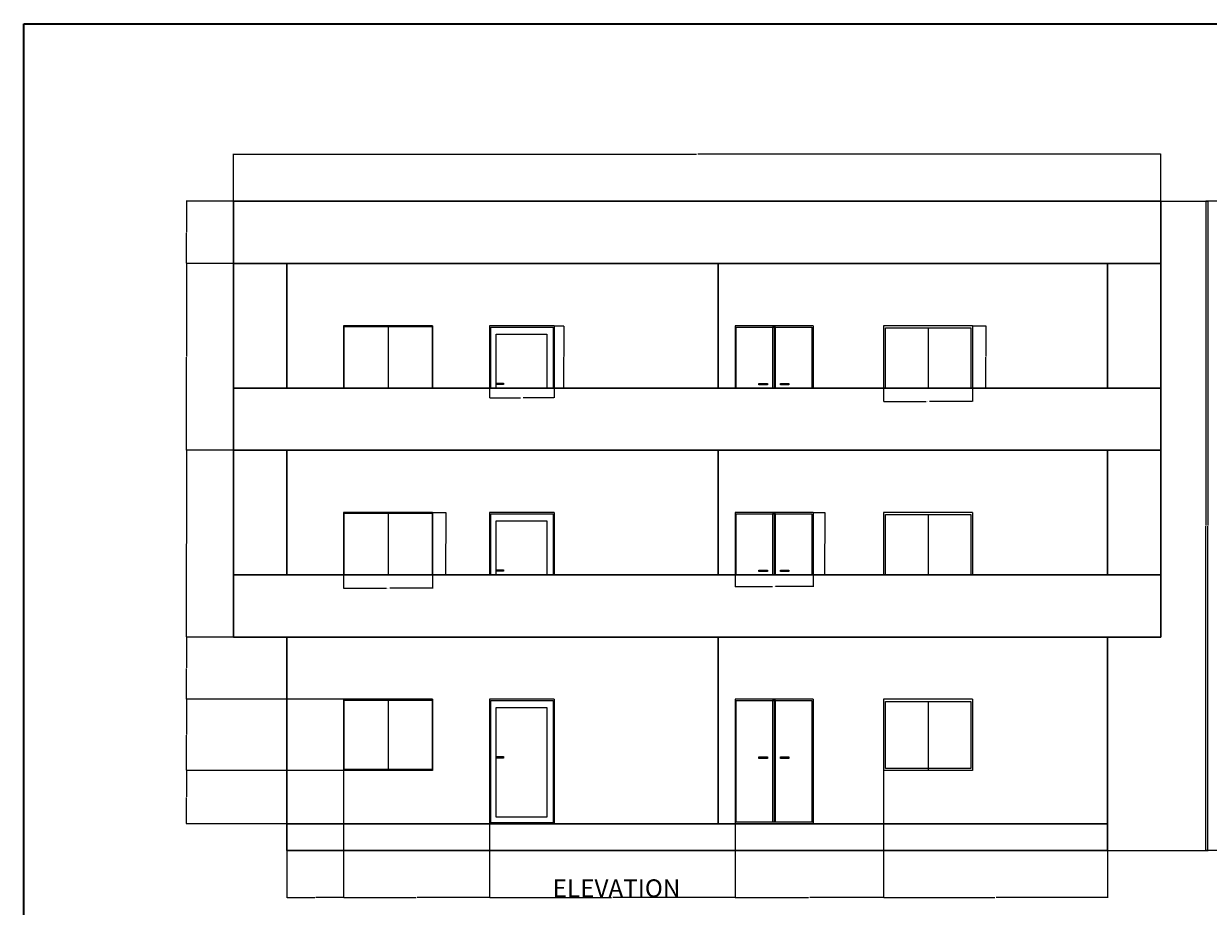
# Model space of a CAD drawing. Units: inches. Extents: x 2014 to 3678, y 870 to 2323.
# Tile 3 of 7: x 2014 to 2813, y 1728 to 2323. Entities that reach past the tile are written whole.
import ezdxf

# ---------------------------------------------------------------- set-up
doc = ezdxf.new("R2010")
doc.units = ezdxf.units.IN
for name, color, linetype, lineweight in [('A-ANNO-DIMS', 2, 'Continuous', 18), ('A-ANNO-TEXT', 7, 'Continuous', 18), ('A-ANNO-TTLB', 7, 'Continuous', 35), ('A-ELEV', 7, 'Continuous', 30), ('A-ELEV-DOOR', 3, 'Continuous', 18), ('A-ELEV-GLAZ', 4, 'Continuous', 18)]:
    doc.layers.add(name, color=color, linetype=linetype, lineweight=lineweight)
doc.styles.get("Standard").update_dxf_attribs({"font": 'arial.ttf'})
doc.dimstyles.get("Standard").update_dxf_attribs({"dimtxt": 0.18, "dimasz": 0.18, "dimexe": 0.18, "dimexo": 0.0625, "dimgap": 0.09, "dimtad": 0, "dimtih": 1, "dimtoh": 1, "dimdec": 4, "dimzin": 0, "dimdsep": 46, "dimtxsty": 'Standard', "dimcen": 0.09, "dimadec": 0, "dimazin": 0, "dimtfac": 1, "dimtdec": 4, "dimtofl": 0, "dimtmove": 0, "dimatfit": 3, "dimfxl": 1, "dimtolj": 1, "dimtzin": 0, "dimarcsym": 0})

# ---------------------------------------------------------------- blocks, each defined once
blk = doc.blocks.new('ELEV-BALCONY-DOOR')
for p, q in [((0, 42), (0, 0)), ((43.48, 42), (0, 42)), ((0, 42), (0, 0)), ((43.48, 42), (0, 42)), ((43.48, 42), (43.48, 0)), ((43.48, 42), (43.48, 0))]:
    blk.add_line(p, q)
for points in [[(0.77, 0), (0.77, 41.09), (42.81, 41.09), (42.81, 0)], [(4.43, 0), (4.43, 36.38), (38.55, 36.38), (38.55, 0)]]:
    blk.add_lwpolyline(points)
blk.add_lwpolyline([(4.43, 3.32), (9.34, 3.32), (9.34, 2.33), (4.43, 2.33)], close=True)
blk = doc.blocks.new('ELEV-BALCONY-DOUBLE-DOOR')
for p, q in [((0, 42), (0, 0)), ((52.71, 42), (0, 42)), ((0, 42), (0, 0)), ((52.71, 42), (0, 42)), ((26.3, 41.16), (25.3, 41.16)), ((25.3, 41.16), (25.3, 0)), ((26.3, 41.16), (26.3, 0)), ((27.3, 41.16), (26.3, 41.16)), ((27.3, 0), (27.3, 41.16)), ((52.71, 42), (52.71, 0)), ((52.71, 42), (52.71, 0))]:
    blk.add_line(p, q)
blk.add_lwpolyline([(0.85, 0), (0.85, 41.16), (51.75, 41.16), (51.75, 0)])
for points in [[(16.11, 3.13), (21.78, 3.13), (21.78, 2.12), (16.11, 2.12)], [(30.59, 3.13), (36.26, 3.13), (36.26, 2.12), (30.59, 2.12)]]:
    blk.add_lwpolyline(points, close=True)
blk = doc.blocks.new('ELEV-BALCONY-WIN-WEST')
for p, q in [((0, 42), (0, 0)), ((60, 42), (0, 42)), ((0, 42), (0, 0)), ((60, 42), (0, 42)), ((30, 42), (30, 0)), ((60, 42), (60, 0)), ((60, 42), (60, 0))]:
    blk.add_line(p, q)
blk.add_lwpolyline([(0.47, 0), (0.47, 41.49), (59.63, 41.49), (59.63, 0)])
blk = doc.blocks.new('ELEV-BALCONY-WIN-EAST')
for p, q in [((0, 42), (0, 0)), ((60, 42), (0, 42)), ((0, 42), (0, 0)), ((60, 42), (0, 42)), ((30.07, 40.6), (30.07, 0)), ((60, 42), (60, 0)), ((60, 42), (60, 0))]:
    blk.add_line(p, q)
blk.add_lwpolyline([(1.35, 0), (1.35, 40.6), (58.8, 40.6), (58.8, 0)])
blk = doc.blocks.new('*D72')
at = {"layer": 'A-ANNO-DIMS', "color": 0, "lineweight": -2, "transparency": 16777216}
for p, q in [((2328.3, 2077.46), (2328.3, 2070.82)), ((2328.48, 2071), (2349.1, 2071)), ((2371.59, 2071), (2350.97, 2071)), ((2371.77, 2077.46), (2371.77, 2070.82))]:
    blk.add_line(p, q, dxfattribs=at)
at = {"layer": 'A-ANNO-DIMS', "color": 0, "transparency": 16777216}
for points in [[(2328.48, 2071.03), (2328.48, 2070.97), (2328.3, 2071)], [(2371.59, 2071.03), (2371.59, 2070.97), (2371.77, 2071)]]:
    blk.add_solid(points, dxfattribs=at)
at = {"layer": 'Defpoints', "color": 0, "transparency": 16777216}
for p in [(2328.3, 2077.52), (2371.77, 2077.52), (2371.77, 2071)]:
    blk.add_point(p, dxfattribs=at)
at = {"layer": 'A-ANNO-DIMS', "color": 0, "transparency": 16777216, "insert": (2350.03, 2071), "char_height": 0.18, "attachment_point": 5}
blk.add_mtext('\\A1;DOOR 43 TYP.', dxfattribs=at)
blk = doc.blocks.new('*D73')
at = {"layer": 'A-ANNO-DIMS', "color": 0, "lineweight": -2, "transparency": 16777216}
for p, q in [((2371.84, 2119.52), (2378.47, 2119.52)), ((2378.29, 2119.34), (2378.29, 2098.7)), ((2378.29, 2077.7), (2378.29, 2098.34)), ((2371.84, 2077.52), (2378.47, 2077.52))]:
    blk.add_line(p, q, dxfattribs=at)
at = {"layer": 'A-ANNO-DIMS', "color": 0, "transparency": 16777216}
for points in [[(2378.26, 2119.34), (2378.32, 2119.34), (2378.29, 2119.52)], [(2378.26, 2077.7), (2378.32, 2077.7), (2378.29, 2077.52)]]:
    blk.add_solid(points, dxfattribs=at)
at = {"layer": 'Defpoints', "color": 0, "transparency": 16777216}
for p in [(2371.77, 2119.52), (2378.29, 2119.52), (2371.77, 2077.52)]:
    blk.add_point(p, dxfattribs=at)
at = {"layer": 'A-ANNO-DIMS', "color": 0, "transparency": 16777216, "insert": (2378.29, 2098.52), "char_height": 0.18, "attachment_point": 5}
blk.add_mtext('\\A1;42 TYP.', dxfattribs=at)
blk = doc.blocks.new('*D74')
at = {"layer": 'A-ANNO-DIMS', "color": 0, "lineweight": -2, "transparency": 16777216}
for p, q in [((2493.87, 1951.46), (2493.87, 1943.44)), ((2546.59, 1951.46), (2546.59, 1943.44)), ((2494.05, 1943.62), (2519.21, 1943.62)), ((2546.41, 1943.62), (2521.25, 1943.62))]:
    blk.add_line(p, q, dxfattribs=at)
at = {"layer": 'A-ANNO-DIMS', "color": 0, "transparency": 16777216}
for points in [[(2494.05, 1943.65), (2494.05, 1943.59), (2493.87, 1943.62)], [(2546.41, 1943.65), (2546.41, 1943.59), (2546.59, 1943.62)]]:
    blk.add_solid(points, dxfattribs=at)
at = {"layer": 'Defpoints', "color": 0, "transparency": 16777216}
for p in [(2493.87, 1951.52), (2546.59, 1951.52), (2546.59, 1943.62)]:
    blk.add_point(p, dxfattribs=at)
at = {"layer": 'A-ANNO-DIMS', "color": 0, "transparency": 16777216, "insert": (2520.23, 1943.62), "char_height": 0.18, "attachment_point": 5}
blk.add_mtext('\\A1;DOORS 53 TYP.', dxfattribs=at)
blk = doc.blocks.new('*D75')
at = {"layer": 'A-ANNO-DIMS', "color": 0, "lineweight": -2, "transparency": 16777216}
for p, q in [((2546.65, 1993.52), (2554.67, 1993.52)), ((2554.49, 1993.34), (2554.49, 1972.7)), ((2554.49, 1951.7), (2554.49, 1972.34)), ((2546.65, 1951.52), (2554.67, 1951.52))]:
    blk.add_line(p, q, dxfattribs=at)
at = {"layer": 'A-ANNO-DIMS', "color": 0, "transparency": 16777216}
for points in [[(2554.46, 1993.34), (2554.52, 1993.34), (2554.49, 1993.52)], [(2554.46, 1951.7), (2554.52, 1951.7), (2554.49, 1951.52)]]:
    blk.add_solid(points, dxfattribs=at)
at = {"layer": 'Defpoints', "color": 0, "transparency": 16777216}
for p in [(2546.59, 1993.52), (2554.49, 1993.52), (2546.59, 1951.52)]:
    blk.add_point(p, dxfattribs=at)
at = {"layer": 'A-ANNO-DIMS', "color": 0, "transparency": 16777216, "insert": (2554.49, 1972.52), "char_height": 0.18, "attachment_point": 5}
blk.add_mtext('\\A1;42 TYP.', dxfattribs=at)
blk = doc.blocks.new('*D76')
at = {"layer": 'A-ANNO-DIMS', "color": 0, "lineweight": -2, "transparency": 16777216}
for p, q in [((2229.86, 1951.46), (2229.86, 1942.34)), ((2289.86, 1951.46), (2289.86, 1942.34)), ((2230.04, 1942.52), (2258.74, 1942.52)), ((2289.68, 1942.52), (2260.98, 1942.52))]:
    blk.add_line(p, q, dxfattribs=at)
at = {"layer": 'A-ANNO-DIMS', "color": 0, "transparency": 16777216}
for points in [[(2230.04, 1942.55), (2230.04, 1942.49), (2229.86, 1942.52)], [(2289.68, 1942.55), (2289.68, 1942.49), (2289.86, 1942.52)]]:
    blk.add_solid(points, dxfattribs=at)
at = {"layer": 'Defpoints', "color": 0, "transparency": 16777216}
for p in [(2229.86, 1951.52), (2289.86, 1951.52), (2289.86, 1942.52)]:
    blk.add_point(p, dxfattribs=at)
at = {"layer": 'A-ANNO-DIMS', "color": 0, "transparency": 16777216, "insert": (2259.86, 1942.52), "char_height": 0.18, "attachment_point": 5}
blk.add_mtext('\\A1;WINDOW 60 TYP.', dxfattribs=at)
blk = doc.blocks.new('*D77')
at = {"layer": 'A-ANNO-DIMS', "color": 0, "lineweight": -2, "transparency": 16777216}
for p, q in [((2289.92, 1993.52), (2299.04, 1993.52)), ((2298.86, 1993.34), (2298.86, 1972.7)), ((2298.86, 1951.7), (2298.86, 1972.34)), ((2289.92, 1951.52), (2299.04, 1951.52))]:
    blk.add_line(p, q, dxfattribs=at)
at = {"layer": 'A-ANNO-DIMS', "color": 0, "transparency": 16777216}
for points in [[(2298.83, 1993.34), (2298.89, 1993.34), (2298.86, 1993.52)], [(2298.83, 1951.7), (2298.89, 1951.7), (2298.86, 1951.52)]]:
    blk.add_solid(points, dxfattribs=at)
at = {"layer": 'Defpoints', "color": 0, "transparency": 16777216}
for p in [(2289.86, 1993.52), (2298.86, 1993.52), (2289.86, 1951.52)]:
    blk.add_point(p, dxfattribs=at)
at = {"layer": 'A-ANNO-DIMS', "color": 0, "transparency": 16777216, "insert": (2298.86, 1972.52), "char_height": 0.18, "attachment_point": 5}
blk.add_mtext('\\A1;42 TYP.', dxfattribs=at)
blk = doc.blocks.new('*D78')
at = {"layer": 'A-ANNO-DIMS', "color": 0, "lineweight": -2, "transparency": 16777216}
for p, q in [((2594, 2077.46), (2594, 2068.34)), ((2654, 2077.46), (2654, 2068.34)), ((2594.18, 2068.52), (2622.89, 2068.52)), ((2653.82, 2068.52), (2625.12, 2068.52))]:
    blk.add_line(p, q, dxfattribs=at)
at = {"layer": 'A-ANNO-DIMS', "color": 0, "transparency": 16777216}
for points in [[(2594.18, 2068.55), (2594.18, 2068.49), (2594, 2068.52)], [(2653.82, 2068.55), (2653.82, 2068.49), (2654, 2068.52)]]:
    blk.add_solid(points, dxfattribs=at)
at = {"layer": 'Defpoints', "color": 0, "transparency": 16777216}
for p in [(2594, 2077.52), (2654, 2077.52), (2654, 2068.52)]:
    blk.add_point(p, dxfattribs=at)
at = {"layer": 'A-ANNO-DIMS', "color": 0, "transparency": 16777216, "insert": (2624, 2068.52), "char_height": 0.18, "attachment_point": 5}
blk.add_mtext('\\A1;WINDOW 60 TYP.', dxfattribs=at)
blk = doc.blocks.new('*D79')
at = {"layer": 'A-ANNO-DIMS', "color": 0, "lineweight": -2, "transparency": 16777216}
for p, q in [((2654.07, 2119.52), (2663.18, 2119.52)), ((2663, 2119.34), (2663, 2098.7)), ((2663, 2077.7), (2663, 2098.34)), ((2654.07, 2077.52), (2663.18, 2077.52))]:
    blk.add_line(p, q, dxfattribs=at)
at = {"layer": 'A-ANNO-DIMS', "color": 0, "transparency": 16777216}
for points in [[(2662.97, 2119.34), (2663.03, 2119.34), (2663, 2119.52)], [(2662.97, 2077.7), (2663.03, 2077.7), (2663, 2077.52)]]:
    blk.add_solid(points, dxfattribs=at)
at = {"layer": 'Defpoints', "color": 0, "transparency": 16777216}
for p in [(2654, 2119.52), (2663, 2119.52), (2654, 2077.52)]:
    blk.add_point(p, dxfattribs=at)
at = {"layer": 'A-ANNO-DIMS', "color": 0, "transparency": 16777216, "insert": (2663, 2098.52), "char_height": 0.18, "attachment_point": 5}
blk.add_mtext('\\A1;42 TYP.', dxfattribs=at)
blk = doc.blocks.new('*D101')
at = {"layer": 'A-ANNO-DIMS', "color": 0, "lineweight": -2, "transparency": 16777216}
for p, q in [((2155.56, 2203.59), (2155.56, 2235.45)), ((2155.74, 2235.27), (2467.92, 2235.27)), ((2780.88, 2235.27), (2468.71, 2235.27)), ((2781.06, 2203.59), (2781.06, 2235.45))]:
    blk.add_line(p, q, dxfattribs=at)
at = {"layer": 'A-ANNO-DIMS', "color": 0, "transparency": 16777216}
for points in [[(2155.74, 2235.3), (2155.74, 2235.24), (2155.56, 2235.27)], [(2780.88, 2235.3), (2780.88, 2235.24), (2781.06, 2235.27)]]:
    blk.add_solid(points, dxfattribs=at)
at = {"layer": 'Defpoints', "color": 0, "transparency": 16777216}
for p in [(2781.06, 2235.27), (2155.56, 2203.52), (2781.06, 2203.52)]:
    blk.add_point(p, dxfattribs=at)
at = {"layer": 'A-ANNO-DIMS', "color": 0, "transparency": 16777216, "insert": (2468.31, 2235.27), "char_height": 0.18, "attachment_point": 5}
blk.add_mtext('\\A1;625.5', dxfattribs=at)
blk = doc.blocks.new('*D102')
at = {"layer": 'A-ANNO-DIMS', "color": 0, "lineweight": -2, "transparency": 16777216}
for p, q in [((2781.12, 2203.52), (2812.99, 2203.52)), ((2812.81, 2203.34), (2812.81, 1984.71)), ((2812.81, 1765.7), (2812.81, 1984.34)), ((2745.12, 1765.52), (2812.99, 1765.52))]:
    blk.add_line(p, q, dxfattribs=at)
at = {"layer": 'A-ANNO-DIMS', "color": 0, "transparency": 16777216}
for points in [[(2812.78, 2203.34), (2812.84, 2203.34), (2812.81, 2203.52)], [(2812.78, 1765.7), (2812.84, 1765.7), (2812.81, 1765.52)]]:
    blk.add_solid(points, dxfattribs=at)
at = {"layer": 'Defpoints', "color": 0, "transparency": 16777216}
for p in [(2781.06, 2203.52), (2812.81, 2203.52), (2745.06, 1765.52)]:
    blk.add_point(p, dxfattribs=at)
at = {"layer": 'A-ANNO-DIMS', "color": 0, "transparency": 16777216, "insert": (2812.81, 1984.52), "char_height": 0.18, "attachment_point": 5}
blk.add_mtext('\\A1;438', dxfattribs=at)
blk = doc.blocks.new('*D103')
at = {"layer": 'A-ANNO-DIMS', "color": 0, "lineweight": -2, "transparency": 16777216}
for p, q in [((2229.8, 1819.52), (2123.63, 1819.52)), ((2123.81, 1819.34), (2123.81, 1801.71)), ((2123.81, 1783.7), (2123.81, 1801.34)), ((2191.5, 1783.52), (2123.63, 1783.52))]:
    blk.add_line(p, q, dxfattribs=at)
at = {"layer": 'A-ANNO-DIMS', "color": 0, "transparency": 16777216}
for points in [[(2123.78, 1819.34), (2123.84, 1819.34), (2123.81, 1819.52)], [(2123.78, 1783.7), (2123.84, 1783.7), (2123.81, 1783.52)]]:
    blk.add_solid(points, dxfattribs=at)
at = {"layer": 'Defpoints', "color": 0, "transparency": 16777216}
for p in [(2123.81, 1819.52), (2229.86, 1819.52), (2191.56, 1783.52)]:
    blk.add_point(p, dxfattribs=at)
at = {"layer": 'A-ANNO-DIMS', "color": 0, "transparency": 16777216, "insert": (2123.81, 1801.52), "char_height": 0.18, "attachment_point": 5}
blk.add_mtext('\\A1;36', dxfattribs=at)
blk = doc.blocks.new('*D104')
at = {"layer": 'A-ANNO-DIMS', "color": 0, "lineweight": -2, "transparency": 16777216}
for p, q in [((2229.8, 1867.52), (2123.63, 1867.52)), ((2123.81, 1867.34), (2123.81, 1843.71)), ((2123.81, 1819.7), (2123.81, 1843.34)), ((2229.8, 1819.52), (2123.63, 1819.52))]:
    blk.add_line(p, q, dxfattribs=at)
at = {"layer": 'A-ANNO-DIMS', "color": 0, "transparency": 16777216}
for points in [[(2123.78, 1867.34), (2123.84, 1867.34), (2123.81, 1867.52)], [(2123.78, 1819.7), (2123.84, 1819.7), (2123.81, 1819.52)]]:
    blk.add_solid(points, dxfattribs=at)
at = {"layer": 'Defpoints', "color": 0, "transparency": 16777216}
for p in [(2123.81, 1867.52), (2229.86, 1867.52), (2229.86, 1819.52)]:
    blk.add_point(p, dxfattribs=at)
at = {"layer": 'A-ANNO-DIMS', "color": 0, "transparency": 16777216, "insert": (2123.81, 1843.52), "char_height": 0.18, "attachment_point": 5}
blk.add_mtext('\\A1;48', dxfattribs=at)
blk = doc.blocks.new('*D105')
at = {"layer": 'A-ANNO-DIMS', "color": 0, "lineweight": -2, "transparency": 16777216}
for p, q in [((2155.5, 1909.52), (2123.63, 1909.52)), ((2123.81, 1909.34), (2123.81, 1888.7)), ((2123.81, 1867.7), (2123.81, 1888.34)), ((2229.8, 1867.52), (2123.63, 1867.52))]:
    blk.add_line(p, q, dxfattribs=at)
at = {"layer": 'A-ANNO-DIMS', "color": 0, "transparency": 16777216}
for points in [[(2123.78, 1909.34), (2123.84, 1909.34), (2123.81, 1909.52)], [(2123.78, 1867.7), (2123.84, 1867.7), (2123.81, 1867.52)]]:
    blk.add_solid(points, dxfattribs=at)
at = {"layer": 'Defpoints', "color": 0, "transparency": 16777216}
for p in [(2123.81, 1909.52), (2155.56, 1909.52), (2229.86, 1867.52)]:
    blk.add_point(p, dxfattribs=at)
at = {"layer": 'A-ANNO-DIMS', "color": 0, "transparency": 16777216, "insert": (2123.81, 1888.52), "char_height": 0.18, "attachment_point": 5}
blk.add_mtext('\\A1;42', dxfattribs=at)
blk = doc.blocks.new('*D106')
at = {"layer": 'A-ANNO-DIMS', "color": 0, "lineweight": -2, "transparency": 16777216}
for p, q in [((2155.5, 2035.52), (2123.63, 2035.52)), ((2123.81, 2035.34), (2123.81, 1972.71)), ((2123.81, 1909.7), (2123.81, 1972.34)), ((2155.5, 1909.52), (2123.63, 1909.52))]:
    blk.add_line(p, q, dxfattribs=at)
at = {"layer": 'A-ANNO-DIMS', "color": 0, "transparency": 16777216}
for points in [[(2123.78, 2035.34), (2123.84, 2035.34), (2123.81, 2035.52)], [(2123.78, 1909.7), (2123.84, 1909.7), (2123.81, 1909.52)]]:
    blk.add_solid(points, dxfattribs=at)
at = {"layer": 'Defpoints', "color": 0, "transparency": 16777216}
for p in [(2123.81, 2035.52), (2155.56, 2035.52), (2155.56, 1909.52)]:
    blk.add_point(p, dxfattribs=at)
at = {"layer": 'A-ANNO-DIMS', "color": 0, "transparency": 16777216, "insert": (2123.81, 1972.52), "char_height": 0.18, "attachment_point": 5}
blk.add_mtext('\\A1;126', dxfattribs=at)
blk = doc.blocks.new('*D107')
at = {"layer": 'A-ANNO-DIMS', "color": 0, "lineweight": -2, "transparency": 16777216}
for p, q in [((2155.5, 2161.52), (2123.63, 2161.52)), ((2123.81, 2161.34), (2123.81, 2098.71)), ((2123.81, 2035.7), (2123.81, 2098.34)), ((2155.5, 2035.52), (2123.63, 2035.52))]:
    blk.add_line(p, q, dxfattribs=at)
at = {"layer": 'A-ANNO-DIMS', "color": 0, "transparency": 16777216}
for points in [[(2123.78, 2161.34), (2123.84, 2161.34), (2123.81, 2161.52)], [(2123.78, 2035.7), (2123.84, 2035.7), (2123.81, 2035.52)]]:
    blk.add_solid(points, dxfattribs=at)
at = {"layer": 'Defpoints', "color": 0, "transparency": 16777216}
for p in [(2123.81, 2161.52), (2155.56, 2161.52), (2155.56, 2035.52)]:
    blk.add_point(p, dxfattribs=at)
at = {"layer": 'A-ANNO-DIMS', "color": 0, "transparency": 16777216, "insert": (2123.81, 2098.52), "char_height": 0.18, "attachment_point": 5}
blk.add_mtext('\\A1;126', dxfattribs=at)
blk = doc.blocks.new('*D108')
at = {"layer": 'A-ANNO-DIMS', "color": 0, "lineweight": -2, "transparency": 16777216}
for p, q in [((2155.5, 2203.52), (2123.63, 2203.52)), ((2123.81, 2203.34), (2123.81, 2182.7)), ((2123.81, 2161.7), (2123.81, 2182.34)), ((2155.5, 2161.52), (2123.63, 2161.52))]:
    blk.add_line(p, q, dxfattribs=at)
at = {"layer": 'A-ANNO-DIMS', "color": 0, "transparency": 16777216}
for points in [[(2123.78, 2203.34), (2123.84, 2203.34), (2123.81, 2203.52)], [(2123.78, 2161.7), (2123.84, 2161.7), (2123.81, 2161.52)]]:
    blk.add_solid(points, dxfattribs=at)
at = {"layer": 'Defpoints', "color": 0, "transparency": 16777216}
for p in [(2123.81, 2203.52), (2155.56, 2203.52), (2155.56, 2161.52)]:
    blk.add_point(p, dxfattribs=at)
at = {"layer": 'A-ANNO-DIMS', "color": 0, "transparency": 16777216, "insert": (2123.81, 2182.52), "char_height": 0.18, "attachment_point": 5}
blk.add_mtext('\\A1;42', dxfattribs=at)
blk = doc.blocks.new('*D109')
at = {"layer": 'A-ANNO-DIMS', "color": 0, "lineweight": -2, "transparency": 16777216}
for p, q in [((2229.86, 1819.46), (2229.86, 1733.59)), ((2191.56, 1765.46), (2191.56, 1733.59)), ((2191.74, 1733.77), (2210.39, 1733.77)), ((2229.68, 1733.77), (2211.03, 1733.77))]:
    blk.add_line(p, q, dxfattribs=at)
at = {"layer": 'A-ANNO-DIMS', "color": 0, "transparency": 16777216}
for points in [[(2191.74, 1733.8), (2191.74, 1733.74), (2191.56, 1733.77)], [(2229.68, 1733.8), (2229.68, 1733.74), (2229.86, 1733.77)]]:
    blk.add_solid(points, dxfattribs=at)
at = {"layer": 'Defpoints', "color": 0, "transparency": 16777216}
for p in [(2229.86, 1819.52), (2191.56, 1765.52), (2229.86, 1733.77)]:
    blk.add_point(p, dxfattribs=at)
at = {"layer": 'A-ANNO-DIMS', "color": 0, "transparency": 16777216, "insert": (2210.71, 1733.77), "char_height": 0.18, "attachment_point": 5}
blk.add_mtext('\\A1;38.3', dxfattribs=at)
blk = doc.blocks.new('*D110')
at = {"layer": 'A-ANNO-DIMS', "color": 0, "lineweight": -2, "transparency": 16777216}
for p, q in [((2229.86, 1819.46), (2229.86, 1733.59)), ((2328.3, 1783.46), (2328.3, 1733.59)), ((2230.04, 1733.77), (2278.68, 1733.77)), ((2328.12, 1733.77), (2279.47, 1733.77))]:
    blk.add_line(p, q, dxfattribs=at)
at = {"layer": 'A-ANNO-DIMS', "color": 0, "transparency": 16777216}
for points in [[(2230.04, 1733.8), (2230.04, 1733.74), (2229.86, 1733.77)], [(2328.12, 1733.8), (2328.12, 1733.74), (2328.3, 1733.77)]]:
    blk.add_solid(points, dxfattribs=at)
at = {"layer": 'Defpoints', "color": 0, "transparency": 16777216}
for p in [(2229.86, 1819.52), (2328.3, 1783.52), (2328.3, 1733.77)]:
    blk.add_point(p, dxfattribs=at)
at = {"layer": 'A-ANNO-DIMS', "color": 0, "transparency": 16777216, "insert": (2279.08, 1733.77), "char_height": 0.18, "attachment_point": 5}
blk.add_mtext('\\A1;98.44', dxfattribs=at)
blk = doc.blocks.new('*D111')
at = {"layer": 'A-ANNO-DIMS', "color": 0, "lineweight": -2, "transparency": 16777216}
for p, q in [((2328.3, 1783.46), (2328.3, 1733.59)), ((2493.87, 1783.46), (2493.87, 1733.59)), ((2328.48, 1733.77), (2410.63, 1733.77)), ((2493.69, 1733.77), (2411.54, 1733.77))]:
    blk.add_line(p, q, dxfattribs=at)
at = {"layer": 'A-ANNO-DIMS', "color": 0, "transparency": 16777216}
for points in [[(2328.48, 1733.8), (2328.48, 1733.74), (2328.3, 1733.77)], [(2493.69, 1733.8), (2493.69, 1733.74), (2493.87, 1733.77)]]:
    blk.add_solid(points, dxfattribs=at)
at = {"layer": 'Defpoints', "color": 0, "transparency": 16777216}
for p in [(2328.3, 1783.52), (2493.87, 1783.52), (2493.87, 1733.77)]:
    blk.add_point(p, dxfattribs=at)
at = {"layer": 'A-ANNO-DIMS', "color": 0, "transparency": 16777216, "insert": (2411.08, 1733.77), "char_height": 0.18, "attachment_point": 5}
blk.add_mtext('\\A1;165.58', dxfattribs=at)
blk = doc.blocks.new('*D112')
at = {"layer": 'A-ANNO-DIMS', "color": 0, "lineweight": -2, "transparency": 16777216}
for p, q in [((2594, 1819.46), (2594, 1733.59)), ((2493.87, 1783.46), (2493.87, 1733.59)), ((2494.05, 1733.77), (2543.48, 1733.77)), ((2593.82, 1733.77), (2544.39, 1733.77))]:
    blk.add_line(p, q, dxfattribs=at)
at = {"layer": 'A-ANNO-DIMS', "color": 0, "transparency": 16777216}
for points in [[(2494.05, 1733.8), (2494.05, 1733.74), (2493.87, 1733.77)], [(2593.82, 1733.8), (2593.82, 1733.74), (2594, 1733.77)]]:
    blk.add_solid(points, dxfattribs=at)
at = {"layer": 'Defpoints', "color": 0, "transparency": 16777216}
for p in [(2594, 1819.52), (2493.87, 1783.52), (2594, 1733.77)]:
    blk.add_point(p, dxfattribs=at)
at = {"layer": 'A-ANNO-DIMS', "color": 0, "transparency": 16777216, "insert": (2543.94, 1733.77), "char_height": 0.18, "attachment_point": 5}
blk.add_mtext('\\A1;100.13', dxfattribs=at)
blk = doc.blocks.new('*D113')
at = {"layer": 'A-ANNO-DIMS', "color": 0, "lineweight": -2, "transparency": 16777216}
for p, q in [((2594, 1819.46), (2594, 1733.59)), ((2745.06, 1765.46), (2745.06, 1733.59)), ((2594.18, 1733.77), (2669.08, 1733.77)), ((2744.88, 1733.77), (2669.99, 1733.77))]:
    blk.add_line(p, q, dxfattribs=at)
at = {"layer": 'A-ANNO-DIMS', "color": 0, "transparency": 16777216}
for points in [[(2594.18, 1733.8), (2594.18, 1733.74), (2594, 1733.77)], [(2744.88, 1733.8), (2744.88, 1733.74), (2745.06, 1733.77)]]:
    blk.add_solid(points, dxfattribs=at)
at = {"layer": 'Defpoints', "color": 0, "transparency": 16777216}
for p in [(2594, 1819.52), (2745.06, 1765.52), (2745.06, 1733.77)]:
    blk.add_point(p, dxfattribs=at)
at = {"layer": 'A-ANNO-DIMS', "color": 0, "transparency": 16777216, "insert": (2669.53, 1733.77), "char_height": 0.18, "attachment_point": 5}
blk.add_mtext('\\A1;151.06', dxfattribs=at)
blk = doc.blocks.new('*D115')
at = {"layer": 'A-ANNO-DIMS', "color": 0, "lineweight": -2, "transparency": 16777216}
for p, q in [((2848.61, 2203.52), (2811.34, 2203.52)), ((2811.52, 2203.34), (2811.52, 1984.71)), ((2811.52, 1765.7), (2811.52, 1984.34)), ((2848.61, 1765.52), (2811.34, 1765.52))]:
    blk.add_line(p, q, dxfattribs=at)
at = {"layer": 'A-ANNO-DIMS', "color": 0, "transparency": 16777216}
for points in [[(2811.49, 2203.34), (2811.55, 2203.34), (2811.52, 2203.52)], [(2811.49, 1765.7), (2811.55, 1765.7), (2811.52, 1765.52)]]:
    blk.add_solid(points, dxfattribs=at)
at = {"layer": 'Defpoints', "color": 0, "transparency": 16777216}
for p in [(2811.52, 2203.52), (2848.67, 2203.52), (2848.67, 1765.52)]:
    blk.add_point(p, dxfattribs=at)
at = {"layer": 'A-ANNO-DIMS', "color": 0, "transparency": 16777216, "insert": (2811.52, 1984.52), "char_height": 0.18, "attachment_point": 5}
blk.add_mtext('\\A1;438', dxfattribs=at)

msp = doc.modelspace()

# ---------------------------------------------------------------- linework, layer by layer
at = {"layer": 'A-ANNO-TTLB'}
msp.add_lwpolyline([(2014.0556, 2323.3638), (3678.0069, 2323.3638), (3678.0069, 869.855), (2014.0556, 869.855)], close=True, dxfattribs=at)
at = {"layer": 'A-ELEV'}
for p, q in [((2781.0607, 2203.5235), (2155.5607, 2203.5235)), ((2155.5607, 1909.5235), (2155.5607, 2203.5235)), ((2781.0607, 1909.5235), (2781.0607, 2203.5235)), ((2191.5607, 2161.5235), (2155.5607, 2161.5235)), ((2191.5607, 2161.5235), (2191.5607, 2077.5235)), ((2781.0607, 2161.5235), (2191.5607, 2161.5235)), ((2482.4577, 2077.5235), (2482.4577, 2161.5235)), ((2745.0607, 2161.5235), (2745.0607, 2077.5235)), ((2781.0607, 2077.5235), (2155.5607, 2077.5235)), ((2781.0607, 2035.5235), (2155.5607, 2035.5235)), ((2191.5607, 2035.5235), (2191.5607, 1951.5235)), ((2191.5607, 2035.5235), (2191.5607, 2017.5235)), ((2482.4577, 1951.5235), (2482.4577, 2035.5235)), ((2745.0607, 2035.5235), (2745.0607, 1951.5235)), ((2745.0607, 2035.5235), (2745.0607, 2017.5235)), ((2781.0607, 1951.5235), (2155.5607, 1951.5235)), ((2781.0607, 1909.5235), (2155.5607, 1909.5235)), ((2191.5607, 1909.5235), (2191.5607, 1765.5235)), ((2191.5607, 1909.5235), (2191.5607, 1891.5235)), ((2482.4577, 1783.5235), (2482.4577, 1909.5235)), ((2745.0607, 1909.5235), (2745.0607, 1765.5235)), ((2745.0607, 1909.5235), (2745.0607, 1891.5235)), ((2745.0607, 1783.5235), (2191.5607, 1783.5235)), ((2745.0607, 1765.5235), (2191.5607, 1765.5235))]:
    msp.add_line(p, q, dxfattribs=at)
at = {"layer": 'A-ELEV-DOOR'}
for p, q in [((2328.295, 1867.5235), (2328.295, 1783.5235)), ((2371.7733, 1867.5235), (2328.295, 1867.5235)), ((2371.7733, 1867.5235), (2371.7733, 1783.5235)), ((2493.8749, 1867.5235), (2493.8749, 1783.5235)), ((2546.5867, 1867.5235), (2493.8749, 1867.5235)), ((2520.1726, 1866.6843), (2519.1726, 1866.6843)), ((2519.1726, 1866.6843), (2519.1726, 1784.5235)), ((2520.1726, 1866.6843), (2520.1726, 1784.5235)), ((2521.1726, 1866.6843), (2520.1726, 1866.6843)), ((2521.1726, 1784.5235), (2521.1726, 1866.6843)), ((2546.5867, 1867.5235), (2546.5867, 1783.5235)), ((2545.622, 1784.5235), (2494.7232, 1784.5235)), ((2520.1726, 1783.5235), (2521.1726, 1783.5235)), ((2546.5867, 1783.5235), (2546.5867, 1784.5235))]:
    msp.add_line(p, q, dxfattribs=at)
for points in [[(2329.0625, 1866.6083), (2371.1079, 1866.6083), (2371.1079, 1784.1073), (2329.0625, 1784.1073)], [(2332.7217, 1861.9026), (2366.8452, 1861.9026), (2366.8452, 1787.865), (2332.7217, 1787.865)], [(2332.7217, 1828.8477), (2337.6355, 1828.8477), (2337.6355, 1827.8552), (2332.7217, 1827.8552)], [(2509.9838, 1828.6568), (2515.6556, 1828.6568), (2515.6556, 1827.6439), (2509.9838, 1827.6439)], [(2524.4627, 1828.6568), (2530.1345, 1828.6568), (2530.1345, 1827.6439), (2524.4627, 1827.6439)]]:
    msp.add_lwpolyline(points, close=True, dxfattribs=at)
for points in [[(2494.7232, 1784.5235), (2494.7232, 1866.6843), (2545.622, 1866.6843), (2545.622, 1784.5235)], [(2545.622, 1783.5235), (2494.7232, 1783.5235)]]:
    msp.add_lwpolyline(points, dxfattribs=at)
at = {"layer": 'A-ELEV-GLAZ'}
for p, q in [((2229.8595, 1867.5235), (2229.8595, 1819.5235)), ((2289.8595, 1867.5235), (2229.8595, 1867.5235)), ((2259.8595, 1867.5235), (2259.8595, 1819.5235)), ((2289.8595, 1867.5235), (2289.8595, 1819.5235)), ((2594.0046, 1867.5235), (2594.0046, 1819.5235)), ((2654.0046, 1867.5235), (2594.0046, 1867.5235)), ((2624.0791, 1866.119), (2624.0791, 1819.5235)), ((2654.0046, 1867.5235), (2654.0046, 1819.5235)), ((2289.8595, 1819.5235), (2229.8595, 1819.5235)), ((2654.0046, 1819.5235), (2594.0046, 1819.5235))]:
    msp.add_line(p, q, dxfattribs=at)
for points in [[(2230.3252, 1867.0105), (2289.4859, 1867.0105), (2289.4859, 1820.0877), (2230.3252, 1820.0877)], [(2595.3542, 1866.119), (2652.804, 1866.119), (2652.804, 1820.7271), (2595.3542, 1820.7271)]]:
    msp.add_lwpolyline(points, close=True, dxfattribs=at)

# ---------------------------------------------------------------- block references
at = {"layer": 'A-ELEV-DOOR'}
for name, p in [('ELEV-BALCONY-DOOR', (2328.295, 2077.523)), ('ELEV-BALCONY-DOUBLE-DOOR', (2493.875, 2077.523)), ('ELEV-BALCONY-DOOR', (2328.295, 1951.523)), ('ELEV-BALCONY-DOUBLE-DOOR', (2493.875, 1951.523))]:
    msp.add_blockref(name, p, dxfattribs=at)
at = {"layer": 'A-ELEV-GLAZ'}
for name, p in [('ELEV-BALCONY-WIN-WEST', (2229.86, 2077.523)), ('ELEV-BALCONY-WIN-EAST', (2594.005, 2077.523)), ('ELEV-BALCONY-WIN-WEST', (2229.86, 1951.523)), ('ELEV-BALCONY-WIN-EAST', (2594.005, 1951.523))]:
    msp.add_blockref(name, p, dxfattribs=at)

# ---------------------------------------------------------------- texts
at = {"layer": 'A-ANNO-TEXT', "insert": (2370.8846, 1745.9964), "char_height": 12, "attachment_point": 1}
msp.add_mtext_dynamic_manual_height_columns('ELEVATION', width=301.874101, gutter_width=12.5, heights=[0], dxfattribs=at)

# ---------------------------------------------------------------- dimensions: what is measured, and where the dimension line sits
at = {"layer": 'A-ANNO-DIMS'}
for base, p1, p2, override, picture, middle in [((2781.0607, 2235.2735), (2155.5607, 2203.5235), (2781.0607, 2203.5235), {"dimdec": 1, "dimlfac": 1, "dimrnd": 0, "dimzin": 0, "dimdsep": 46, "dimlunit": 2}, '*D101', (2468.3107, 2235.2735)), ((2229.8595, 1733.7735), (2191.5607, 1765.5235), (2229.8595, 1819.5235), {"dimdec": 1, "dimlfac": 1, "dimrnd": 0, "dimzin": 0, "dimdsep": 46, "dimlunit": 2}, '*D109', (2210.7101, 1733.7735)), ((2328.295, 1733.7735), (2229.8595, 1819.5235), (2328.295, 1783.5235), {"dimdec": 2, "dimlfac": 1, "dimrnd": 0, "dimzin": 0, "dimdsep": 46, "dimlunit": 2}, '*D110', (2279.0773, 1733.7735)), ((2594.0046, 1733.7735), (2493.8749, 1783.5235), (2594.0046, 1819.5235), {"dimdec": 2, "dimlfac": 1, "dimrnd": 0, "dimzin": 0, "dimdsep": 46, "dimlunit": 2}, '*D112', (2543.9397, 1733.7735)), ((2745.0607, 1733.7735), (2594.0046, 1819.5235), (2745.0607, 1765.5235), {"dimdec": 2, "dimlfac": 1, "dimrnd": 0, "dimzin": 0, "dimdsep": 46, "dimlunit": 2}, '*D113', (2669.5326, 1733.7735)), ((2493.8749, 1733.7735), (2328.295, 1783.5235), (2493.8749, 1783.5235), {"dimdec": 2, "dimlfac": 1, "dimrnd": 0, "dimzin": 0, "dimdsep": 46, "dimlunit": 2}, '*D111', (2411.085, 1733.7735))]:
    dim = msp.add_linear_dim(base=base, p1=p1, p2=p2, dimstyle='Standard', override=override, dxfattribs=at)
    dim.commit()
    dim.dimension.update_dxf_attribs({"geometry": picture, "text_midpoint": middle})
for base, p1, p2, picture, middle in [((2123.8107, 2203.5235), (2155.5607, 2161.5235), (2155.5607, 2203.5235), '*D108', (2123.8107, 2182.5235)), ((2812.8107, 2203.5235), (2745.0607, 1765.5235), (2781.0607, 2203.5235), '*D102', (2812.8107, 1984.5235)), ((2811.5218, 2203.5235), (2848.6718, 1765.5235), (2848.6718, 2203.5235), '*D115', (2811.5218, 1984.5235)), ((2123.8107, 2161.5235), (2155.5607, 2035.5235), (2155.5607, 2161.5235), '*D107', (2123.8107, 2098.5235)), ((2123.8107, 2035.5235), (2155.5607, 1909.5235), (2155.5607, 2035.5235), '*D106', (2123.8107, 1972.5235)), ((2123.8107, 1909.5235), (2229.8595, 1867.5235), (2155.5607, 1909.5235), '*D105', (2123.8107, 1888.5235)), ((2123.8107, 1867.5235), (2229.8595, 1819.5235), (2229.8595, 1867.5235), '*D104', (2123.8107, 1843.5235)), ((2123.8107, 1819.5235), (2191.5607, 1783.5235), (2229.8595, 1819.5235), '*D103', (2123.8107, 1801.5235))]:
    dim = msp.add_linear_dim(base=base, p1=p1, p2=p2, angle=90, dimstyle='Standard', override={"dimdec": 0, "dimlfac": 1, "dimrnd": 0, "dimzin": 0, "dimdsep": 46, "dimlunit": 2}, dxfattribs=at)
    dim.commit()
    dim.dimension.update_dxf_attribs({"geometry": picture, "text_midpoint": middle})
for base, p1, p2, picture, middle in [((2378.295, 2119.5235), (2371.7733, 2077.5235), (2371.7733, 2119.5235), '*D73', (2378.295, 2098.5235)), ((2663.0046, 2119.5235), (2654.0046, 2077.5235), (2654.0046, 2119.5235), '*D79', (2663.0046, 2098.5235)), ((2298.8595, 1993.5235), (2289.8595, 1951.5235), (2289.8595, 1993.5235), '*D77', (2298.8595, 1972.5235)), ((2554.4935, 1993.5235), (2546.5867, 1951.5235), (2546.5867, 1993.5235), '*D75', (2554.4935, 1972.5235))]:
    dim = msp.add_linear_dim(base=base, p1=p1, p2=p2, angle=90, text='<> TYP.', dimstyle='Standard', override={"dimdec": 0, "dimlfac": 1, "dimrnd": 0, "dimzin": 0, "dimdsep": 46, "dimlunit": 2}, dxfattribs=at)
    dim.commit()
    dim.dimension.update_dxf_attribs({"geometry": picture, "text_midpoint": middle})
for base, p1, p2, text, picture, middle in [((2371.7733, 2071.0018), (2328.295, 2077.5235), (2371.7733, 2077.5235), 'DOOR <> TYP.', '*D72', (2350.0341, 2071.0018)), ((2654.0046, 2068.5235), (2594.0046, 2077.5235), (2654.0046, 2077.5235), 'WINDOW <> TYP.', '*D78', (2624.0046, 2068.5235)), ((2289.8595, 1942.5235), (2229.8595, 1951.5235), (2289.8595, 1951.5235), 'WINDOW <> TYP.', '*D76', (2259.8595, 1942.5235)), ((2546.5867, 1943.6167), (2493.8749, 1951.5235), (2546.5867, 1951.5235), 'DOORS <> TYP.', '*D74', (2520.2308, 1943.6167))]:
    dim = msp.add_linear_dim(base=base, p1=p1, p2=p2, text=text, dimstyle='Standard', override={"dimdec": 0, "dimlfac": 1, "dimrnd": 0, "dimzin": 0, "dimdsep": 46, "dimlunit": 2}, dxfattribs=at)
    dim.commit()
    dim.dimension.update_dxf_attribs({"geometry": picture, "text_midpoint": middle})

doc.saveas('drawing.dxf')
